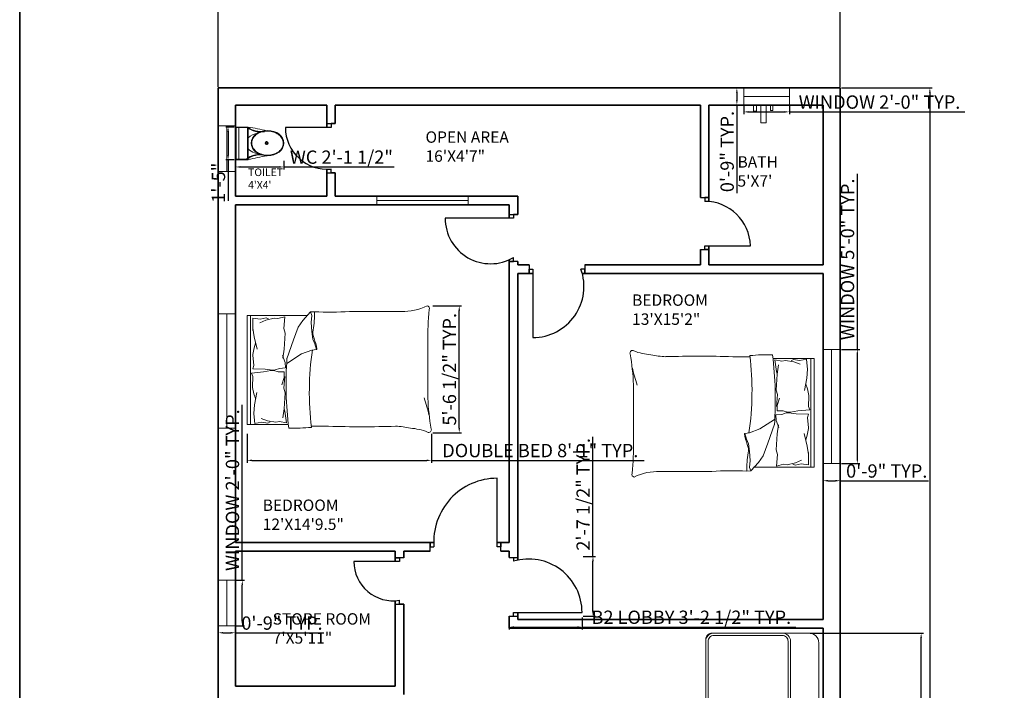
# Model space of a CAD drawing. Units: inches. Extents: x 1863 to 2938, y 1238 to 2492.
# Tile 9 of 12: x 1863 to 2381, y 1760 to 2112. Entities that reach past the tile are written whole.
import ezdxf

# ---------------------------------------------------------------- set-up
doc = ezdxf.new("R2010")
doc.units = ezdxf.units.IN
for name, color, linetype, lineweight in [('A-ANNO-DIMS', 2, 'Continuous', 18), ('A-ANNO-TTLB', 7, 'Continuous', 35), ('A-AREA-IDEN', 7, 'Continuous', 18), ('A-DOOR', 3, 'Continuous', 25), ('A-FLOR-FIXT', 9, 'Continuous', 18), ('A-FURN', 8, 'Continuous', 18), ('A-GLAZ', 4, 'Continuous', 18), ('A-WALL', 7, 'Continuous', 35)]:
    doc.layers.add(name, color=color, linetype=linetype, lineweight=lineweight)
doc.styles.get("Standard").update_dxf_attribs({"font": 'arial.ttf'})
doc.dimstyles.new('ISO-25', dxfattribs={"dimtxt": 7, "dimasz": 2.5, "dimexe": 1.25, "dimexo": 0.625, "dimtad": 1, "dimdec": 0, "dimlunit": 3, "dimtxsty": 'Standard', "dimcen": 2.5, "dimadec": 0, "dimazin": 0, "dimtfac": 1, "dimtdec": 0, "dimtmove": 0, "dimatfit": 3, "dimfxl": 1, "dimarcsym": 0})

# ---------------------------------------------------------------- blocks, each defined once
blk = doc.blocks.new('*D2')
at = {"layer": 'A-ANNO-DIMS', "color": 0, "lineweight": -2, "transparency": 16777216}
for p, q in [((1967.64, 2077.19), (1967.64, 2118.26)), ((2294.64, 2077.19), (2294.64, 2118.26)), ((1970.14, 2117.01), (2292.14, 2117.01))]:
    blk.add_line(p, q, dxfattribs=at)
at = {"layer": 'A-ANNO-DIMS', "color": 0, "transparency": 16777216}
for points in [[(1970.14, 2117.43), (1970.14, 2116.59), (1967.64, 2117.01)], [(2292.14, 2117.43), (2292.14, 2116.59), (2294.64, 2117.01)]]:
    blk.add_solid(points, dxfattribs=at)
at = {"layer": 'Defpoints', "color": 0, "transparency": 16777216}
for p in [(2294.64, 2117.01), (1967.64, 2076.56), (2294.64, 2076.56)]:
    blk.add_point(p, dxfattribs=at)
at = {"layer": 'A-ANNO-DIMS', "color": 0, "transparency": 16777216, "insert": (2131.14, 2121.21), "char_height": 7, "attachment_point": 5}
blk.add_mtext('27\'-3"', dxfattribs=at)
blk = doc.blocks.new('*D3')
at = {"layer": 'A-ANNO-DIMS', "color": 0, "lineweight": -2, "transparency": 16777216}
for p, q in [((2295.26, 2076.56), (2343.03, 2076.56)), ((2341.78, 2074.06), (2341.78, 1342.06)), ((2295.26, 1339.56), (2343.03, 1339.56))]:
    blk.add_line(p, q, dxfattribs=at)
at = {"layer": 'A-ANNO-DIMS', "color": 0, "transparency": 16777216}
for points in [[(2341.36, 2074.06), (2342.2, 2074.06), (2341.78, 2076.56)], [(2341.36, 1342.06), (2342.2, 1342.06), (2341.78, 1339.56)]]:
    blk.add_solid(points, dxfattribs=at)
at = {"layer": 'Defpoints', "color": 0, "transparency": 16777216}
for p in [(2294.64, 2076.56), (2294.64, 1339.56), (2341.78, 1339.56)]:
    blk.add_point(p, dxfattribs=at)
at = {"layer": 'A-ANNO-DIMS', "color": 0, "transparency": 16777216, "insert": (2337.58, 1708.06), "char_height": 7, "attachment_point": 5, "rotation": 90}
blk.add_mtext('61\'-5"', dxfattribs=at)
blk = doc.blocks.new('A$C31115884')
for p, q in [((283, 498), (223, 498)), ((258, 466), (258, 523)), ((0, 200), (0, 0)), ((520, 200), (0, 200)), ((10, 190), (10, 10)), ((510, 190), (10, 190)), ((510, 10), (510, 190)), ((520, 0), (520, 200)), ((510, 54), (0, 54)), ((10, 10), (510, 10)), ((0, 0), (520, 0))]:
    blk.add_line(p, q)
blk.add_circle((256, 496), 23.6)
for centre, radius, start, end in [((2778, -205), 2807, 165.4549, 171.7133), ((3237, 905), 2807, 188.2867, 194.5451), ((-295, 403), 365, 324.2091, 9.3499), ((-295, 403), 375, 324.2091, 9.3499), ((384, 406), 293, 190.2774, 224.1564), ((139, 406), 293, 315.8436, 2.6563), ((806, 403), 375, 179.2036, 215.7909), ((806, 403), 365, 170.6501, 215.7909)]:
    blk.add_arc(centre, radius, start, end)
blk.add_ellipse((256, 510), major_axis=(0, -261), ratio=0.772727)
blk.add_open_spline([(256, 259), (263, 259), (270, 260), (288, 262), (299, 265), (320, 273), (330, 278), (350, 291), (360, 299), (378, 316), (386, 326), (402, 347), (409, 358), (421, 383), (427, 395), (436, 422), (440, 436), (445, 465), (447, 480), (448, 509), (448, 524), (445, 553), (443, 568), (436, 596), (432, 610), (422, 636), (416, 649), (402, 672), (395, 683), (379, 703), (370, 712), (351, 728), (341, 735), (321, 746), (310, 751), (289, 757), (278, 759), (256, 761), (245, 761), (223, 757), (212, 754), (191, 746), (181, 741), (161, 728), (151, 720), (133, 703), (125, 693), (110, 672), (103, 660), (90, 636), (85, 623), (76, 596), (72, 582), (67, 553), (66, 538), (64, 509), (65, 494), (68, 465), (70, 450), (77, 422), (81, 408), (91, 382), (97, 370), (111, 346), (118, 335), (135, 316), (144, 307), (162, 291), (172, 284), (193, 273), (203, 269), (225, 262), (236, 260), (250, 259), (253, 259), (256, 259)], degree=3, knots=[0, 0, 0, 0, 0.110105, 0.110105, 0.285049, 0.285049, 0.459994, 0.459994, 0.634938, 0.634938, 0.809882, 0.809882, 0.984827, 0.984827, 1.159771, 1.159771, 1.334715, 1.334715, 1.50966, 1.50966, 1.684604, 1.684604, 1.859549, 1.859549, 2.034493, 2.034493, 2.209437, 2.209437, 2.384382, 2.384382, 2.559326, 2.559326, 2.73427, 2.73427, 2.909215, 2.909215, 3.084159, 3.084159, 3.259103, 3.259103, 3.434048, 3.434048, 3.608992, 3.608992, 3.783936, 3.783936, 3.958881, 3.958881, 4.133825, 4.133825, 4.30877, 4.30877, 4.483714, 4.483714, 4.658658, 4.658658, 4.833603, 4.833603, 5.008547, 5.008547, 5.183491, 5.183491, 5.358436, 5.358436, 5.53338, 5.53338, 5.708324, 5.708324, 5.883269, 5.883269, 6.058213, 6.058213, 6.233158, 6.233158, 6.283185, 6.283185, 6.283185, 6.283185])
blk = doc.blocks.new('DOOR-24-TOILET')
for p, q in [((24, 23.86), (0, 23.86)), ((21.75, 25.86), (26.25, 25.86)), ((26.25, 25.86), (24, 25.86)), ((24, 25.86), (24, 23.86)), ((21.75, 0), (26.25, 0)), ((24, 0), (24, 2)), ((26.25, 0), (24, 0))]:
    blk.add_line(p, q)
blk.add_arc((21.96, 23.86), 21.96, 180, 275.3383)
blk = doc.blocks.new('DOOR-36-BED1-REAR')
for p, q in [((33.75, 25.94), (38.25, 25.94)), ((38.25, 25.94), (36, 25.94)), ((36, 25.94), (36, 23.94)), ((36, 23.94), (0, 23.94)), ((38.25, 1.26), (33.75, 1.26)), ((33.75, 1.26), (36, 1.26)), ((36, 1.26), (36, 3.26))]:
    blk.add_line(p, q)
blk.add_arc((23.94, 23.94), 23.94, 180, 300.2375)
blk = doc.blocks.new('DOOR-24-BATH')
for p, q in [((0, 27.38), (4.5, 27.38)), ((4.5, 27.38), (2.25, 27.38)), ((2.25, 27.38), (2.25, 25.38)), ((0, 0), (4.5, 0)), ((2.25, 0), (2.25, 2)), ((2.25, 2), (26.25, 2)), ((4.5, 0), (2.25, 0))]:
    blk.add_line(p, q)
blk.add_arc((2.25, 1.37), 24.01, 1.5021, 90)
blk = doc.blocks.new('DOOR-36-BED2-REAR')
for p, q in [((0, 38.25), (0, 33.75)), ((29.25, 38.25), (29.25, 33.75)), ((0, 33.75), (0, 36)), ((0, 36), (2, 36)), ((2, 36), (2, 0)), ((29.25, 36), (27.25, 36)), ((29.25, 33.75), (29.25, 36))]:
    blk.add_line(p, q)
blk.add_arc((2, 26.86), 26.86, 270, 19.9084)
blk = doc.blocks.new('DOOR-36-BED2-LOBBY')
for p, q in [((0, 30.86), (4.5, 30.86)), ((2.25, 30.86), (2.25, 28.86)), ((0, 0), (4.5, 0)), ((2.25, 0), (2.25, 2)), ((2.25, 2), (38.25, 2))]:
    blk.add_line(p, q)
blk.add_arc((10.23, 2), 28.02, 0, 106.5507)
blk = doc.blocks.new('DOOR-24-STORE')
for p, q in [((24, 22.39), (0, 22.39)), ((26.25, 24.39), (21.75, 24.39)), ((21.75, 24.39), (24, 24.39)), ((24, 24.39), (24, 22.39)), ((24, 0), (24, 2)), ((21.75, 0), (26.25, 0)), ((26.25, 0), (24, 0))]:
    blk.add_line(p, q)
blk.add_arc((20.66, 22.39), 20.66, 180, 279.3111)
blk = doc.blocks.new('DOOR-36-BED1-LOBBY')
for p, q in [((35.21, 2.25), (35.21, 38.25)), ((0, 0), (0, 4.5)), ((0, 4.5), (0, 2.25)), ((0, 2.25), (2, 2.25)), ((37.21, 2.25), (35.21, 2.25)), ((37.21, 0), (37.21, 4.5)), ((37.21, 4.5), (37.21, 2.25))]:
    blk.add_line(p, q)
blk.add_arc((35.21, 4.93), 33.32, 90, 184.6101)
blk = doc.blocks.new('WIN-24')
for p, q in [((0, 24), (9, 24)), ((9, 24), (4.5, 24)), ((4.5, 24), (4.5, 0)), ((4.5, 0), (0, 0)), ((0, 0), (9, 0))]:
    blk.add_line(p, q)
blk = doc.blocks.new('WIN-48')
for p, q in [((0, 4.5), (0, 0)), ((0, 0), (0, 2.25)), ((0, 2.25), (48, 2.25)), ((48, 2.25), (48, 4.5)), ((48, 4.5), (48, 0))]:
    blk.add_line(p, q)
blk = doc.blocks.new('WIN-60')
for p, q in [((0, 60), (9, 60)), ((9, 60), (4.5, 60)), ((4.5, 60), (4.5, 0)), ((4.5, 0), (0, 0)), ((0, 0), (9, 0))]:
    blk.add_line(p, q)
blk = doc.blocks.new('WIN-24-STORE')
for p, q in [((0, 24), (9, 24)), ((9, 24), (4.5, 24)), ((4.5, 24), (4.5, 0)), ((9, 0), (0, 0)), ((4.5, 0), (9, 0))]:
    blk.add_line(p, q)
blk = doc.blocks.new('BED-DOUBLE')
for p, q in [((33.26, 63.38), (29.37, 58.94)), ((35.36, 63.48), (33.26, 63.38, 4.64)), ((34.01, 61.54), (33.26, 63.38)), ((0, 61.46), (31.9, 61.46)), ((0, 4.17), (0, 61.46)), ((1.84, 4.17), (1.84, 61.46)), ((3.07, 60.08), (2.95, 53.6)), ((3.07, 60.08), (6.91, 59.62)), ((9.9, 59.12), (6.69, 57.7)), ((6.91, 59.62), (10, 60.34)), ((14.18, 60.08), (9.9, 59.12)), ((10, 60.34), (11.25, 59.72)), ((16.11, 59.85), (14.18, 60.08)), ((19.87, 60.78), (16.11, 59.85)), ((19.38, 54.63), (19.87, 60.78)), ((29.37, 58.94), (26.77, 55.41)), ((33.63, 57.83), (34.01, 61.54)), ((34.01, 53.18), (33.63, 57.83)), ((2.95, 53.6), (3.05, 54.8)), ((3.05, 54.8), (3.68, 50.25)), ((20.05, 52.28), (19.38, 54.63)), ((19.54, 43.88), (20.05, 52.28)), ((26.77, 55.41), (24.36, 48.73)), ((34.56, 49.1), (34.01, 53.18)), ((3.68, 50.25), (5.3, 43.75)), ((4.4, 47), (3.69, 44.52)), ((24.36, 48.73), (20.84, 38.73)), ((35.68, 46.69), (34.56, 49.1)), ((36.42, 43.72), (35.68, 46.69)), ((95, 18.06), (95, 47.57)), ((3.69, 44.52), (3.04, 41.01)), ((18.74, 39.04), (19.54, 43.88)), ((28.62, 41.3), (34.01, 43.34)), ((34.01, 43.34), (36.42, 43.72)), ((3.04, 41.01), (3.07, 40.62)), ((3.07, 40.62), (3.57, 35.31)), ((20.07, 36.87), (18.53, 40.55)), ((20.25, 33.93), (20.07, 36.87)), ((20.84, 36.28), (28.62, 41.3)), ((2.24, 31.15), (8.66, 31.84)), ((2.94, 29.42), (2.24, 31.15)), ((3.57, 35.31), (2.99, 33.54)), ((2.99, 33.54), (9.43, 33.25)), ((8.66, 31.84), (12.47, 32.54)), ((9.43, 33.25), (13.28, 32.8)), ((12.47, 32.54), (14.03, 32.54)), ((13.28, 32.8), (14.84, 32.89)), ((14.03, 32.54), (16.28, 31.84)), ((14.84, 32.89), (17.04, 33.73)), ((16.28, 31.84), (19.5, 31.84)), ((17.04, 33.73), (20.25, 33.93)), ((19.5, 31.84), (19.5, 28.9)), ((2.76, 24.09), (2.94, 29.42)), ((19.5, 28.9), (18.19, 25.13)), ((19.38, 23.24), (19.87, 29.39)), ((2.76, 23.7), (2.76, 24.09)), ((3.63, 20.24), (2.76, 23.7)), ((3.98, 14.52), (5.19, 21.1)), ((20.05, 20.89), (19.38, 23.24)), ((19.54, 12.49), (20.05, 20.89)), ((4.5, 17.81), (3.63, 20.24)), ((3.63, 9.93), (3.98, 14.52)), ((18.74, 7.65), (19.54, 12.49)), ((19.54, 12.49), (19.92, 11.13)), ((19.92, 11.13), (20.79, 5.02)), ((3.61, 9.81), (3.63, 9.93)), ((4, 4.68), (3.61, 9.81)), ((3.98, 4.67), (7.79, 5.36)), ((10.74, 6.06), (7.44, 7.27)), ((7.79, 5.36), (10.91, 4.84)), ((15.07, 5.36), (10.74, 6.06)), ((10.91, 4.84), (12.12, 5.54)), ((16.98, 5.71), (15.07, 5.36)), ((20.79, 5.02), (16.98, 5.71)), ((21.71, 4.17), (0, 4.17))]:
    blk.add_line(p, q)
for centre, radius, start, end in [((-7.98, 61.54), 43.38, 349.8763, 2.5657), ((43.54, 218.51), 155.25, 266.9791, 273.8365), ((81.31, -5405.34), 5469.02, 90.00217, 90.28689), ((82.32, 91.3), 27.65, 267.4714, 296.4681), ((94.55, 65.23), 1.32, 332.6588, 86.02), ((254.49, 49.34), 159.5, 174.4998, 180.6351), ((42.04, 52.44), 7.46, 168.6608, 203.7384), ((1.78, 37.35), 35.55, 10.6617, 19.8806), ((187.4, 21.29), 154.68, 171.7845, 186.9006), ((36.49, 43.92), 0.221, 250.2464, 1.1377), ((218.26, 25.61), 197.77, 176.0865, 186.7821), ((-28.43, -20.64), 127.63, 13.3832, 17.7053), ((240.78, 25.69), 145.97, 182.9958, 189.4091), ((24.09, 102.1), 99.87, 268.7218, 275.604), ((37.37, -200.58), 203.94, 88.4762, 91.0082), ((60.68, 581.23), 578.22, 268.22771, 271.71854), ((77.34, -32.25), 35.53, 76.0648, 88.9113), ((84.25, -25.96), 28.25, 67.9751, 86.652), ((95.57, 1.31), 1.31, 236.1736, 23.4781)]:
    blk.add_arc(centre, radius, start, end)
blk = doc.blocks.new('*D24')
at = {"layer": 'A-ANNO-DIMS', "color": 0, "lineweight": -2, "transparency": 16777216}
for p, q in [((2303.64, 1939.02), (2303.64, 2031.35)), ((2295.26, 1939.02), (2304.89, 1939.02)), ((2303.64, 1881.52), (2303.64, 1936.52)), ((2295.26, 1879.02), (2304.89, 1879.02))]:
    blk.add_line(p, q, dxfattribs=at)
at = {"layer": 'A-ANNO-DIMS', "color": 0, "transparency": 16777216}
for points in [[(2303.22, 1936.52), (2304.06, 1936.52), (2303.64, 1939.02)], [(2303.22, 1881.52), (2304.06, 1881.52), (2303.64, 1879.02)]]:
    blk.add_solid(points, dxfattribs=at)
at = {"layer": 'Defpoints', "color": 0, "transparency": 16777216}
for p in [(2294.64, 1939.02), (2303.64, 1939.02), (2294.64, 1879.02)]:
    blk.add_point(p, dxfattribs=at)
at = {"layer": 'A-ANNO-DIMS', "color": 0, "transparency": 16777216, "insert": (2299.39, 1986.43), "char_height": 7, "attachment_point": 5, "rotation": 90}
blk.add_mtext('WINDOW 5\'-0" TYP.', dxfattribs=at)
blk = doc.blocks.new('*D25')
at = {"layer": 'A-ANNO-DIMS', "color": 0, "lineweight": -2, "transparency": 16777216}
for p, q in [((2285.64, 1878.39), (2285.64, 1868.77)), ((2294.64, 1878.39), (2294.64, 1868.77)), ((2288.14, 1870.02), (2292.14, 1870.02)), ((2294.64, 1870.02), (2341.06, 1870.02))]:
    blk.add_line(p, q, dxfattribs=at)
at = {"layer": 'A-ANNO-DIMS', "color": 0, "transparency": 16777216}
for points in [[(2288.14, 1870.43), (2288.14, 1869.6), (2285.64, 1870.02)], [(2292.14, 1870.43), (2292.14, 1869.6), (2294.64, 1870.02)]]:
    blk.add_solid(points, dxfattribs=at)
at = {"layer": 'Defpoints', "color": 0, "transparency": 16777216}
for p in [(2285.64, 1879.02), (2294.64, 1879.02), (2294.64, 1870.02)]:
    blk.add_point(p, dxfattribs=at)
at = {"layer": 'A-ANNO-DIMS', "color": 0, "transparency": 16777216, "insert": (2319.1, 1874.22), "char_height": 7, "attachment_point": 5}
blk.add_mtext('0\'-9" TYP.', dxfattribs=at)
blk = doc.blocks.new('*D26')
at = {"layer": 'A-ANNO-DIMS', "color": 0, "lineweight": -2, "transparency": 16777216}
for p, q in [((2243.9, 2066.94), (2243.9, 2062.71)), ((2267.9, 2066.94), (2267.9, 2062.71)), ((2246.4, 2063.96), (2265.4, 2063.96)), ((2267.9, 2063.96), (2360.22, 2063.96))]:
    blk.add_line(p, q, dxfattribs=at)
at = {"layer": 'A-ANNO-DIMS', "color": 0, "transparency": 16777216}
for points in [[(2246.4, 2064.38), (2246.4, 2063.55), (2243.9, 2063.96)], [(2265.4, 2064.38), (2265.4, 2063.55), (2267.9, 2063.96)]]:
    blk.add_solid(points, dxfattribs=at)
at = {"layer": 'Defpoints', "color": 0, "transparency": 16777216}
for p in [(2243.9, 2067.56), (2267.9, 2067.56), (2267.9, 2063.96)]:
    blk.add_point(p, dxfattribs=at)
at = {"layer": 'A-ANNO-DIMS', "color": 0, "transparency": 16777216, "insert": (2315.31, 2068.21), "char_height": 7, "attachment_point": 5}
blk.add_mtext('WINDOW 2\'-0" TYP.', dxfattribs=at)
blk = doc.blocks.new('*D27')
at = {"layer": 'A-ANNO-DIMS', "color": 0, "lineweight": -2, "transparency": 16777216}
for p, q in [((2243.27, 2076.56), (2239.05, 2076.56)), ((2240.3, 2074.06), (2240.3, 2070.06)), ((2243.27, 2067.56), (2239.05, 2067.56)), ((2240.3, 2067.56), (2240.3, 2021.14))]:
    blk.add_line(p, q, dxfattribs=at)
at = {"layer": 'A-ANNO-DIMS', "color": 0, "transparency": 16777216}
for points in [[(2239.88, 2074.06), (2240.71, 2074.06), (2240.3, 2076.56)], [(2239.88, 2070.06), (2240.71, 2070.06), (2240.3, 2067.56)]]:
    blk.add_solid(points, dxfattribs=at)
at = {"layer": 'Defpoints', "color": 0, "transparency": 16777216}
for p in [(2243.9, 2076.56), (2240.3, 2067.56), (2243.9, 2067.56)]:
    blk.add_point(p, dxfattribs=at)
at = {"layer": 'A-ANNO-DIMS', "color": 0, "transparency": 16777216, "insert": (2236.1, 2043.1), "char_height": 7, "attachment_point": 5, "rotation": 90}
blk.add_mtext('0\'-9" TYP.', dxfattribs=at)
blk = doc.blocks.new('*D30')
at = {"layer": 'A-ANNO-DIMS', "color": 0, "lineweight": -2, "transparency": 16777216}
for p, q in [((1980.24, 1817.66), (1980.24, 1909.99)), ((1977.26, 1817.66), (1981.49, 1817.66)), ((1980.24, 1796.16), (1980.24, 1815.16)), ((1977.26, 1793.66), (1981.49, 1793.66))]:
    blk.add_line(p, q, dxfattribs=at)
at = {"layer": 'A-ANNO-DIMS', "color": 0, "transparency": 16777216}
for points in [[(1979.82, 1815.16), (1980.66, 1815.16), (1980.24, 1817.66)], [(1979.82, 1796.16), (1980.66, 1796.16), (1980.24, 1793.66)]]:
    blk.add_solid(points, dxfattribs=at)
at = {"layer": 'Defpoints', "color": 0, "transparency": 16777216}
for p in [(1976.64, 1817.66), (1980.24, 1817.66), (1976.64, 1793.66)]:
    blk.add_point(p, dxfattribs=at)
at = {"layer": 'A-ANNO-DIMS', "color": 0, "transparency": 16777216, "insert": (1975.99, 1865.07), "char_height": 7, "attachment_point": 5, "rotation": 90}
blk.add_mtext('WINDOW 2\'-0" TYP.', dxfattribs=at)
blk = doc.blocks.new('*D31')
at = {"layer": 'A-ANNO-DIMS', "color": 0, "lineweight": -2, "transparency": 16777216}
for p, q in [((1967.64, 1793.03), (1967.64, 1788.81)), ((1976.64, 1793.03), (1976.64, 1788.81)), ((1970.14, 1790.06), (1974.14, 1790.06)), ((1976.64, 1790.06), (2023.06, 1790.06))]:
    blk.add_line(p, q, dxfattribs=at)
at = {"layer": 'A-ANNO-DIMS', "color": 0, "transparency": 16777216}
for points in [[(1970.14, 1790.48), (1970.14, 1789.64), (1967.64, 1790.06)], [(1974.14, 1790.48), (1974.14, 1789.64), (1976.64, 1790.06)]]:
    blk.add_solid(points, dxfattribs=at)
at = {"layer": 'Defpoints', "color": 0, "transparency": 16777216}
for p in [(1967.64, 1793.66), (1976.64, 1793.66), (1976.64, 1790.06)]:
    blk.add_point(p, dxfattribs=at)
at = {"layer": 'A-ANNO-DIMS', "color": 0, "transparency": 16777216, "insert": (2001.1, 1794.26), "char_height": 7, "attachment_point": 5}
blk.add_mtext('0\'-9" TYP.', dxfattribs=at)
blk = doc.blocks.new('*D34')
at = {"layer": 'A-ANNO-DIMS', "color": 0, "lineweight": -2, "transparency": 16777216}
for p, q in [((1982.77, 1894.65), (1982.77, 1879.48)), ((2079.77, 1894.65), (2079.77, 1879.48)), ((1985.27, 1880.73), (2077.27, 1880.73)), ((2079.77, 1880.73), (2191.6, 1880.73))]:
    blk.add_line(p, q, dxfattribs=at)
at = {"layer": 'A-ANNO-DIMS', "color": 0, "transparency": 16777216}
for points in [[(1985.27, 1881.14), (1985.27, 1880.31), (1982.77, 1880.73)], [(2077.27, 1881.14), (2077.27, 1880.31), (2079.77, 1880.73)]]:
    blk.add_solid(points, dxfattribs=at)
at = {"layer": 'Defpoints', "color": 0, "transparency": 16777216}
for p in [(1982.77, 1895.28), (2079.77, 1895.28), (2079.77, 1880.73)]:
    blk.add_point(p, dxfattribs=at)
at = {"layer": 'A-ANNO-DIMS', "color": 0, "transparency": 16777216, "insert": (2136.93, 1884.97), "char_height": 7, "attachment_point": 5}
blk.add_mtext('DOUBLE BED 8\'-1" TYP.', dxfattribs=at)
blk = doc.blocks.new('*D35')
at = {"layer": 'A-ANNO-DIMS', "color": 0, "lineweight": -2, "transparency": 16777216}
for p, q in [((2080.4, 1961.93), (2095.57, 1961.93)), ((2094.32, 1897.78), (2094.32, 1959.43)), ((2080.4, 1895.28), (2095.57, 1895.28))]:
    blk.add_line(p, q, dxfattribs=at)
at = {"layer": 'A-ANNO-DIMS', "color": 0, "transparency": 16777216}
for points in [[(2093.9, 1959.43), (2094.74, 1959.43), (2094.32, 1961.93)], [(2093.9, 1897.78), (2094.74, 1897.78), (2094.32, 1895.28)]]:
    blk.add_solid(points, dxfattribs=at)
at = {"layer": 'Defpoints', "color": 0, "transparency": 16777216}
for p in [(2079.77, 1961.93), (2094.32, 1961.93), (2079.77, 1895.28)]:
    blk.add_point(p, dxfattribs=at)
at = {"layer": 'A-ANNO-DIMS', "color": 0, "transparency": 16777216, "insert": (2090.08, 1928.6), "char_height": 7, "attachment_point": 5, "rotation": 90}
blk.add_mtext('5\'-6 1/2" TYP.', dxfattribs=at)
blk = doc.blocks.new('*D36')
at = {"layer": 'A-ANNO-DIMS', "color": 0, "lineweight": -2, "transparency": 16777216}
for p, q in [((1976.64, 2038.2), (1976.64, 2033.75)), ((1979.14, 2035), (1999.62, 2035)), ((2002.12, 2038.2), (2002.12, 2033.75)), ((2002.12, 2035), (2060.08, 2035))]:
    blk.add_line(p, q, dxfattribs=at)
at = {"layer": 'A-ANNO-DIMS', "color": 0, "transparency": 16777216}
for points in [[(1979.14, 2035.42), (1979.14, 2034.58), (1976.64, 2035)], [(1999.62, 2035.42), (1999.62, 2034.58), (2002.12, 2035)]]:
    blk.add_solid(points, dxfattribs=at)
at = {"layer": 'Defpoints', "color": 0, "transparency": 16777216}
for p in [(1976.64, 2038.82), (2002.12, 2038.82), (2002.12, 2035)]:
    blk.add_point(p, dxfattribs=at)
at = {"layer": 'A-ANNO-DIMS', "color": 0, "transparency": 16777216, "insert": (2032.35, 2039.24), "char_height": 7, "attachment_point": 5}
blk.add_mtext('WC 2\'-1 1/2"', dxfattribs=at)
blk = doc.blocks.new('*D37')
at = {"layer": 'A-ANNO-DIMS', "color": 0, "lineweight": -2, "transparency": 16777216}
for p, q in [((1976.01, 2056.01), (1971.57, 2056.01)), ((1972.82, 2053.51), (1972.82, 2041.32)), ((1976.01, 2038.82), (1971.57, 2038.82)), ((1972.82, 2038.82), (1972.82, 2017.12))]:
    blk.add_line(p, q, dxfattribs=at)
at = {"layer": 'A-ANNO-DIMS', "color": 0, "transparency": 16777216}
for points in [[(1972.4, 2053.51), (1973.23, 2053.51), (1972.82, 2056.01)], [(1972.4, 2041.32), (1973.23, 2041.32), (1972.82, 2038.82)]]:
    blk.add_solid(points, dxfattribs=at)
at = {"layer": 'Defpoints', "color": 0, "transparency": 16777216}
for p in [(1976.64, 2056.01), (1972.82, 2038.82), (1976.64, 2038.82)]:
    blk.add_point(p, dxfattribs=at)
at = {"layer": 'A-ANNO-DIMS', "color": 0, "transparency": 16777216, "insert": (1968.62, 2026.72), "char_height": 7, "attachment_point": 5, "rotation": 90}
blk.add_mtext('1\'-5"', dxfattribs=at)
blk = doc.blocks.new('*D48')
at = {"layer": 'A-ANNO-DIMS', "color": 0, "lineweight": -2, "transparency": 16777216}
for p, q in [((2120.64, 1798.18), (2120.64, 1791.81)), ((2158.89, 1798.18), (2158.89, 1791.81)), ((2123.14, 1793.06), (2156.39, 1793.06)), ((2158.89, 1793.06), (2271.32, 1793.06))]:
    blk.add_line(p, q, dxfattribs=at)
at = {"layer": 'A-ANNO-DIMS', "color": 0, "transparency": 16777216}
for points in [[(2123.14, 1793.48), (2123.14, 1792.65), (2120.64, 1793.06)], [(2156.39, 1793.48), (2156.39, 1792.65), (2158.89, 1793.06)]]:
    blk.add_solid(points, dxfattribs=at)
at = {"layer": 'Defpoints', "color": 0, "transparency": 16777216}
for p in [(2120.64, 1798.8), (2158.89, 1798.8), (2158.89, 1793.06)]:
    blk.add_point(p, dxfattribs=at)
at = {"layer": 'A-ANNO-DIMS', "color": 0, "transparency": 16777216, "insert": (2216.35, 1797.31), "char_height": 7, "attachment_point": 5}
blk.add_mtext('B2 LOBBY 3\'-2 1/2" TYP.', dxfattribs=at)
blk = doc.blocks.new('*D49')
at = {"layer": 'A-ANNO-DIMS', "color": 0, "lineweight": -2, "transparency": 16777216}
for p, q in [((2164.63, 1830.18), (2164.63, 1893.03)), ((2159.51, 1830.18), (2165.88, 1830.18)), ((2164.63, 1801.3), (2164.63, 1827.68)), ((2159.51, 1798.8), (2165.88, 1798.8))]:
    blk.add_line(p, q, dxfattribs=at)
at = {"layer": 'A-ANNO-DIMS', "color": 0, "transparency": 16777216}
for points in [[(2164.21, 1827.68), (2165.04, 1827.68), (2164.63, 1830.18)], [(2164.21, 1801.3), (2165.04, 1801.3), (2164.63, 1798.8)]]:
    blk.add_solid(points, dxfattribs=at)
at = {"layer": 'Defpoints', "color": 0, "transparency": 16777216}
for p in [(2158.89, 1830.18), (2164.63, 1830.18), (2158.89, 1798.8)]:
    blk.add_point(p, dxfattribs=at)
at = {"layer": 'A-ANNO-DIMS', "color": 0, "transparency": 16777216, "insert": (2160.38, 1862.85), "char_height": 7, "attachment_point": 5, "rotation": 90}
blk.add_mtext('2\'-7 1/2" TYP.', dxfattribs=at)
blk = doc.blocks.new('*D59')
at = {"layer": 'A-ANNO-DIMS', "color": 0, "lineweight": -2, "transparency": 16777216}
for p, q in [((2278.91, 1789.89), (2338.44, 1789.89)), ((2337.19, 1622.48), (2337.19, 1787.39)), ((2278.91, 1619.98), (2338.44, 1619.98))]:
    blk.add_line(p, q, dxfattribs=at)
at = {"layer": 'A-ANNO-DIMS', "color": 0, "transparency": 16777216}
for points in [[(2336.77, 1787.39), (2337.61, 1787.39), (2337.19, 1789.89)], [(2336.77, 1622.48), (2337.61, 1622.48), (2337.19, 1619.98)]]:
    blk.add_solid(points, dxfattribs=at)
at = {"layer": 'Defpoints', "color": 0, "transparency": 16777216}
for p in [(2278.29, 1789.89), (2337.19, 1789.89), (2278.29, 1619.98)]:
    blk.add_point(p, dxfattribs=at)
at = {"layer": 'A-ANNO-DIMS', "color": 0, "transparency": 16777216, "insert": (2333.05, 1704.93), "char_height": 7, "attachment_point": 5, "rotation": 90}
blk.add_mtext('14\'-2"', dxfattribs=at)

msp = doc.modelspace()

# ---------------------------------------------------------------- linework, layer by layer
at = {"layer": 'A-ANNO-TTLB'}
msp.add_lwpolyline([(1863.2, 2492.19), (2938.41, 2492.19), (2938.41, 1253.47), (1863.2, 1253.47)], close=True, dxfattribs=at)
at = {"layer": 'A-FLOR-FIXT'}
for points in [[(2250.66, 2067.56), (2249.09, 2067.56), (2249.09, 2064.41), (2250.66, 2064.41)], [(2255.64, 2067.56), (2252.97, 2067.56), (2252.97, 2058.15), (2255.64, 2058.15)], [(2259.22, 2067.56), (2257.94, 2067.56), (2257.94, 2064.61), (2259.22, 2064.61)]]:
    msp.add_lwpolyline(points, close=True, dxfattribs=at)
at = {"layer": 'A-FURN'}
for points in [[(2228.16, 1732.54), (2264.27, 1732.54, 0.414214), (2268.52, 1736.79), (2268.52, 1785.64, 0.414214), (2264.27, 1789.89), (2228.16, 1789.89, 0.414214), (2223.92, 1785.64), (2223.92, 1736.79, 0.414214)], [(2228.16, 1733.82), (2264.27, 1733.82, 0.414214), (2267.24, 1736.79), (2267.24, 1785.64, 0.414214), (2264.27, 1788.61), (2228.16, 1788.61, 0.414214), (2225.19, 1785.64), (2225.19, 1736.79, 0.414214)]]:
    msp.add_lwpolyline(points, format="xyb", close=True, dxfattribs=at)
at = {"layer": 'A-FURN', "ltscale": 0.03}
msp.add_lwpolyline([(2223.92, 1673.88), (2223.92, 1623.37, 0.414214), (2227.31, 1619.98), (2278.29, 1619.98, 0.414214), (2283.38, 1625.07), (2283.38, 1784.79, 0.414214), (2278.29, 1789.89), (2227.31, 1789.89, 0.414214), (2223.92, 1786.49), (2223.92, 1735.98, 0.414214), (2227.31, 1732.58, -1), (2227.31, 1732.5, 0.414214), (2223.92, 1729.1), (2223.92, 1680.76, 0.414214), (2227.31, 1677.36, -1), (2227.31, 1677.28, 0.414214)], format="xyb", close=True, dxfattribs=at)
at = {"layer": 'A-WALL'}
for p, q in [((1967.64, 2076.56), (1967.64, 1339.56)), ((1967.64, 2076.56), (1967.64, 1339.56)), ((1967.64, 2076.56), (2294.64, 2076.56)), ((2294.64, 2076.56), (2294.64, 1495.56)), ((1976.64, 2067.56), (2024.64, 2067.56)), ((1976.64, 2067.56), (1976.64, 2019.56)), ((2024.64, 2067.56), (2024.64, 2055.79)), ((2029.14, 2067.56), (2029.14, 2057.79)), ((2029.14, 2067.56), (2221.14, 2067.56)), ((2221.14, 2067.56), (2221.14, 2018.92)), ((2225.64, 2067.56), (2225.64, 2016.81)), ((2225.64, 2067.56), (2285.64, 2067.56)), ((2285.64, 2067.56), (2285.64, 1983.56)), ((2024.64, 2033.84), (2024.64, 2019.56)), ((2029.14, 2031.93), (2029.14, 2019.56)), ((1976.64, 2019.56), (2024.64, 2019.56)), ((2029.14, 2019.56), (2125.14, 2019.56)), ((2125.14, 2019.56), (2125.14, 2010.05)), ((1976.64, 2015.06), (2120.64, 2015.06)), ((1976.64, 2015.06), (1976.64, 1837.56)), ((2120.64, 2015.06), (2120.64, 2008.05)), ((2225.64, 1993.54), (2225.64, 1983.56)), ((2221.14, 1991.54), (2221.14, 1983.56)), ((2120.64, 1986.21), (2120.64, 1837.56)), ((2125.14, 1985.37), (2125.14, 1983.56)), ((2125.14, 1983.56), (2131.04, 1983.56)), ((2160.3, 1983.56), (2221.14, 1983.56)), ((2225.64, 1983.56), (2285.64, 1983.56)), ((2125.14, 1979.06), (2133.04, 1979.06)), ((2125.14, 1979.06), (2125.14, 1828.23)), ((2159, 1979.06), (2285.64, 1979.06)), ((2285.64, 1979.06), (2285.64, 1797.06)), ((1976.64, 1837.56), (2079.04, 1837.56)), ((1976.64, 1833.06), (2060.64, 1833.06)), ((1976.64, 1833.06), (1976.64, 1762.06)), ((2060.64, 1833.06), (2060.64, 1827.54)), ((2060.64, 1833.06), (2060.64, 1827.54)), ((2065.14, 1837.56), (2080.93, 1837.56)), ((2065.14, 1833.06), (2065.14, 1829.54)), ((2065.14, 1833.06), (2079.04, 1833.06)), ((2065.14, 1833.06), (2065.14, 1829.54)), ((2114.25, 1837.56), (2120.64, 1837.56)), ((2116.25, 1833.06), (2120.64, 1833.06)), ((2120.64, 1833.06), (2120.64, 1829.66)), ((2060.64, 1806.91), (2060.64, 1762.06)), ((2060.64, 1806.91), (2060.64, 1762.06)), ((2065.14, 1805.16), (2065.14, 1762.06)), ((2065.14, 1805.16), (2065.14, 1762.06)), ((2120.64, 1798.8), (2120.64, 1792.56)), ((2125.14, 1800.8), (2125.14, 1797.06)), ((2125.14, 1797.06), (2285.64, 1797.06)), ((2125.14, 1792.56), (2120.64, 1792.56)), ((2125.14, 1792.56), (2285.64, 1792.56)), ((2285.64, 1792.56), (2285.64, 1576.56)), ((1976.64, 1762.06), (2060.64, 1762.06)), ((2065.14, 1762.06), (2065.14, 1757.56))]:
    msp.add_line(p, q, dxfattribs=at)

# ---------------------------------------------------------------- block references
at = {"layer": 'A-DOOR'}
for name, p in [('DOOR-24-TOILET', (2002.89, 2031.93)), ('DOOR-24-BATH', (2221.14, 1991.54)), ('DOOR-36-BED1-REAR', (2086.89, 1984.11)), ('DOOR-36-BED2-REAR', (2131.04, 1945.31)), ('DOOR-36-BED1-LOBBY', (2079.04, 1833.06)), ('DOOR-24-STORE', (2038.89, 1805.16)), ('DOOR-36-BED2-LOBBY', (2120.64, 1798.8))]:
    msp.add_blockref(name, p, dxfattribs=at)
at = {"layer": 'A-FLOR-FIXT', "xscale": 0.0330640103915726, "yscale": 0.0330640103915726, "zscale": 0.0330640103915726, "rotation": 269.9999999999999}
msp.add_blockref('A$C31115884', (1976.64, 2056.01), dxfattribs=at)
at = {"layer": 'A-FURN'}
msp.add_blockref('BED-DOUBLE', (1982.77, 1895.38), dxfattribs=at)
at = {"layer": 'A-FURN', "rotation": 180}
msp.add_blockref('BED-DOUBLE', (2280.98, 1938.52), dxfattribs=at)
at = {"layer": 'A-GLAZ', "rotation": 270.0000000000037}
msp.add_blockref('WIN-24', (2243.9, 2076.56), dxfattribs=at)
at = {"layer": 'A-GLAZ'}
for name, p in [('WIN-24', (1967.64, 2032.59)), ('WIN-48', (2051.05, 2015.06)), ('WIN-60', (1967.64, 1897.7)), ('WIN-60', (2285.64, 1879.02)), ('WIN-24-STORE', (1967.64, 1793.66))]:
    msp.add_blockref(name, p, dxfattribs=at)

# ---------------------------------------------------------------- texts
at = {"layer": 'A-AREA-IDEN', "attachment_point": 1}
for s, width, insert, char_height in [('OPEN AREA\\P16\'X4\'7"', 144.5449, (2076.59, 2053.71), 6), ("BATH\\P5'X7'", 88.1872, (2240.64, 2040.65), 6), ("TOILET\\P4'X4'", 73.2869, (1983.31, 2034.21), 4), ('BEDROOM\\P13\'X15\'2" ', 118.3193, (2185.22, 1967.98), 6), ('BEDROOM\\P12\'X14\'9.5"', 188.1575, (1990.99, 1860.13), 6), ('STORE ROOM\\P7\'X5\'11"', 156.4831, (1996.22, 1800.35), 6)]:
    msp.add_mtext_dynamic_manual_height_columns(s, width=width, gutter_width=12.5, heights=[0], dxfattribs=dict(at, insert=insert, char_height=char_height))

# ---------------------------------------------------------------- dimensions: what is measured, and where the dimension line sits
at = {"layer": 'A-ANNO-DIMS'}
dim = msp.add_linear_dim(base=(2294.64, 2117.01), p1=(1967.64, 2076.56), p2=(2294.64, 2076.56), dimstyle='ISO-25', override={"dimclrd": 0, "dimclre": 0, "dimclrt": 0}, dxfattribs=at)
dim.commit()
dim.dimension.update_dxf_attribs({"geometry": '*D2', "text_midpoint": (2131.14, 2121.21)})
for base, p1, p2, angle, text, picture, middle in [((2267.9, 2063.96), (2243.9, 2067.56), (2267.9, 2067.56), 0, 'WINDOW <> TYP.', '*D26', (2315.31, 2068.21)), ((2240.3, 2067.56), (2243.9, 2076.56), (2243.9, 2067.56), 270, '<> TYP.', '*D27', (2236.1, 2043.1)), ((2303.64, 1939.02), (2294.64, 1879.02), (2294.64, 1939.02), 90, 'WINDOW <> TYP.', '*D24', (2299.39, 1986.43)), ((2094.3208, 1961.9288), (2079.7709, 1895.2773), (2079.7709, 1961.9288), 90, '<> TYP.', '*D35', (2090.0764, 1928.6031)), ((1980.24, 1817.66), (1976.64, 1793.66), (1976.64, 1817.66), 90, 'WINDOW <> TYP.', '*D30', (1975.99, 1865.07)), ((2164.63, 1830.18), (2158.89, 1798.8), (2158.89, 1830.18), 90, '<> TYP.', '*D49', (2160.38, 1862.85))]:
    dim = msp.add_linear_dim(base=base, p1=p1, p2=p2, angle=angle, text=text, dimstyle='ISO-25', override={"dimdec": 1, "dimlfac": 1, "dimrnd": 0, "dimzin": 1, "dimdsep": 46, "dimlunit": 4, "dimfrac": 2}, dxfattribs=at)
    dim.commit()
    dim.dimension.update_dxf_attribs({"geometry": picture, "text_midpoint": middle})
for base, p1, p2, angle, override, picture, middle in [((2341.78, 1339.56), (2294.64, 2076.56), (2294.64, 1339.56), 90, {"dimclrd": 0, "dimclre": 0, "dimclrt": 0}, '*D3', (2337.58, 1708.06)), ((1972.82, 2038.82), (1976.64, 2056.01), (1976.64, 2038.82), 270, {"dimdec": 1, "dimlfac": 1, "dimrnd": 0, "dimzin": 1, "dimdsep": 46, "dimlunit": 4, "dimfrac": 2}, '*D37', (1968.62, 2026.72)), ((2337.19, 1789.89), (2278.29, 1619.98), (2278.29, 1789.89), 90, {"dimdec": 1, "dimlfac": 1, "dimrnd": 0, "dimzin": 1, "dimdsep": 46, "dimlunit": 4, "dimfrac": 2}, '*D59', (2333.05, 1704.93))]:
    dim = msp.add_linear_dim(base=base, p1=p1, p2=p2, angle=angle, dimstyle='ISO-25', override=override, dxfattribs=at)
    dim.commit()
    dim.dimension.update_dxf_attribs({"geometry": picture, "text_midpoint": middle})
for base, p1, p2, text, picture, middle in [((2002.12, 2035), (1976.64, 2038.82), (2002.12, 2038.82), 'WC <>', '*D36', (2032.35, 2039.24)), ((2079.77, 1880.73), (1982.77, 1895.28), (2079.77, 1895.28), 'DOUBLE BED <> TYP.', '*D34', (2136.93, 1884.97)), ((2294.64, 1870.02), (2285.64, 1879.02), (2294.64, 1879.02), '<> TYP.', '*D25', (2319.1, 1874.22)), ((2158.88960651, 1793.06451647), (2120.63960651, 1798.80201647), (2158.88960651, 1798.80201647), 'B2 LOBBY <> TYP.', '*D48', (2216.35294212, 1797.31366381)), ((1976.64, 1790.06), (1967.64, 1793.66), (1976.64, 1793.66), '<> TYP.', '*D31', (2001.1, 1794.26))]:
    dim = msp.add_linear_dim(base=base, p1=p1, p2=p2, text=text, dimstyle='ISO-25', override={"dimdec": 1, "dimlfac": 1, "dimrnd": 0, "dimzin": 1, "dimdsep": 46, "dimlunit": 4, "dimfrac": 2}, dxfattribs=at)
    dim.commit()
    dim.dimension.update_dxf_attribs({"geometry": picture, "text_midpoint": middle})

doc.saveas('drawing.dxf')
